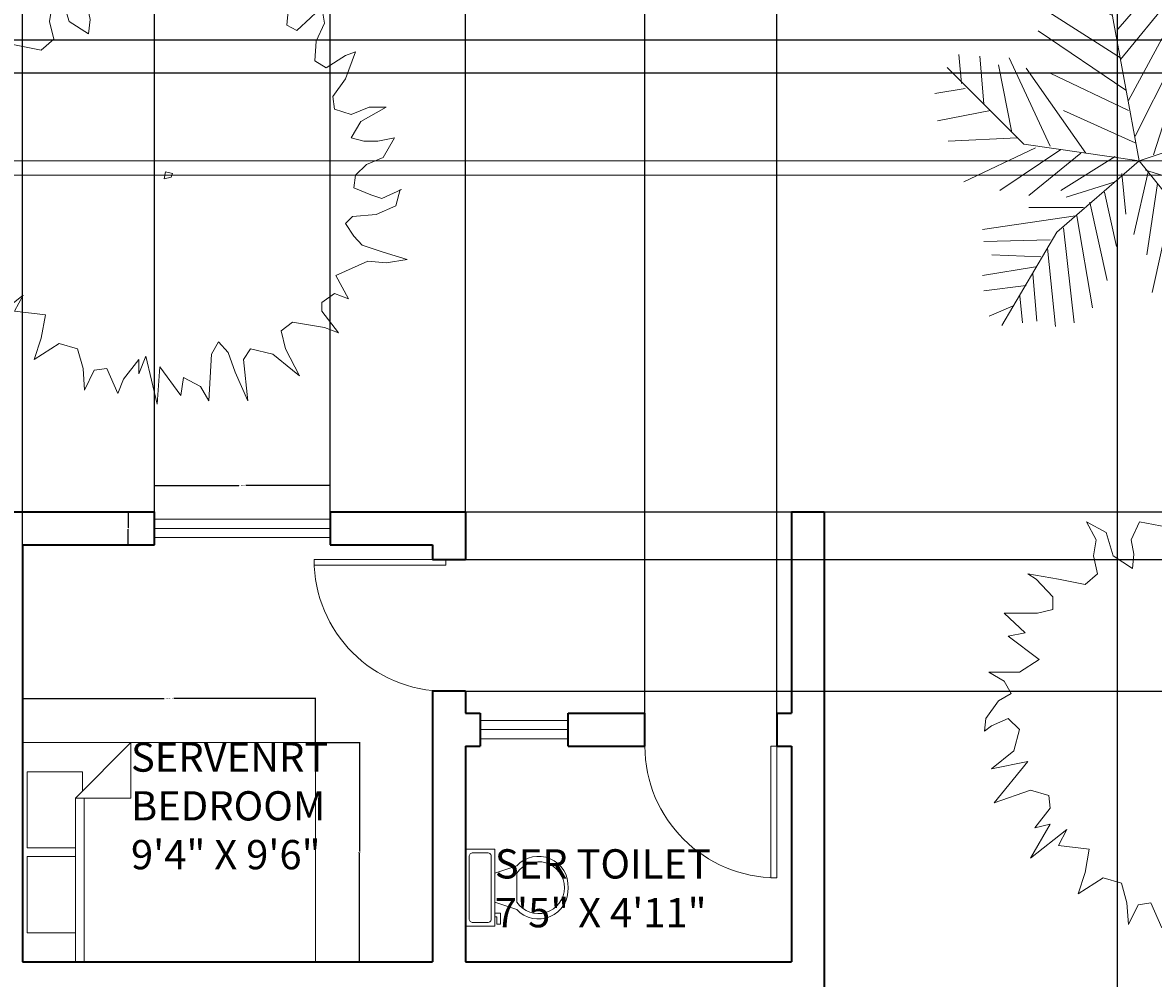
# Model space of a CAD drawing. Units: inches. Extents: x -4843 to -3402, y -164 to 3629.
# Tile 20 of 22: x -4303 to -3994, y 893 to 1154. Entities that reach past the tile are written whole.
import ezdxf

# ---------------------------------------------------------------- set-up
doc = ezdxf.new("R2010")
doc.units = ezdxf.units.IN
for name, color, linetype, lineweight in [('A-ANNO-DIMS', 2, 'Continuous', 18), ('A-AREA-IDEN', 2, 'Continuous', 18), ('C-PROP', 7, 'Continuous', 25), ('doors', 2, 'Continuous', 18), ('furniture', 6, 'Continuous', 18), ('L-PLNT-EDGE', 7, 'Continuous', 18), ('PLANTS', 3, 'Continuous', 13), ('toilets', 5, 'Continuous', 18), ('walls', 7, 'Continuous', 35), ('windows', 1, 'Continuous', 18)]:
    doc.layers.add(name, color=color, linetype=linetype, lineweight=lineweight)
doc.styles.get("Standard").update_dxf_attribs({"font": 'arial.ttf'})
doc.dimstyles.get("Standard").update_dxf_attribs({"dimtxt": 0.18, "dimasz": 0.18, "dimexe": 0.18, "dimexo": 0.0625, "dimgap": 0.09, "dimtad": 0, "dimtih": 1, "dimtoh": 1, "dimdec": 4, "dimzin": 0, "dimdsep": 46, "dimtxsty": 'Standard', "dimcen": 0.09, "dimadec": 0, "dimazin": 0, "dimtfac": 1, "dimtdec": 4, "dimtofl": 0, "dimtmove": 0, "dimatfit": 3, "dimfxl": 1, "dimtolj": 1, "dimtzin": 0, "dimarcsym": 0})

# ---------------------------------------------------------------- blocks, each defined once
blk = doc.blocks.new('window 2')
at = {"layer": 'windows'}
for p, q in [((0, 8.18), (24, 8.18)), ((0, 5.68), (24, 5.68)), ((0, 3.18), (24, 3.18))]:
    blk.add_line(p, q, dxfattribs=at)
for points in [[(0, 10.18), (0, 1.18)], [(24, 1.18), (24, 10.18)]]:
    blk.add_lwpolyline(points, dxfattribs=at)
blk = doc.blocks.new('window 4')
at = {"layer": 'windows'}
for p, q in [((0, 7), (48, 7)), ((0, 4.5), (48, 4.5)), ((0, 2), (48, 2))]:
    blk.add_line(p, q, dxfattribs=at)
for points in [[(0, 0), (0, 9)], [(48, 9), (48, 0)]]:
    blk.add_lwpolyline(points, dxfattribs=at)
blk = doc.blocks.new('*U8')
for p, q in [((0, 0), (0, -6)), ((-40, 0), (-40, -6))]:
    blk.add_line(p, q)
blk.add_lwpolyline([(0, 0), (0, 40), (-1.75, 40), (-1.75, 0)], close=True)
blk.add_arc((0, 0), 40, 90, 180)
blk = doc.blocks.new('*U9')
for p, q in [((-40, 0), (-40, 6)), ((0, 0), (0, 6))]:
    blk.add_line(p, q)
blk.add_lwpolyline([(0, 0), (0, -40), (-1.75, -40), (-1.75, 0)], close=True)
blk.add_arc((0, 0), 40, 180, 270)
blk = doc.blocks.new('Bed - Queen')
for p, q in [((0, -80.00003), (0, 0)), ((0, 0), (59.99999, 0)), ((59.99999, 0), (59.99999, -80.00003)), ((7.99999, -1.2), (28.79998, -1.2)), ((7.99999, -14.4), (7.99999, -1.2)), ((28.79998, -1.2), (28.79998, -14.4)), ((31.19999, -1.2), (51.99999, -1.2)), ((31.19999, -14.4), (31.19999, -1.2)), ((51.99999, -1.2), (51.99999, -16.4)), ((0, -14.4), (44.8, -14.4)), ((59.99999, -29.6), (44.8, -14.4)), ((44.8, -14.4), (44.8, -29.6)), ((44.8, -16.8), (0, -16.8)), ((51.99999, -16.4), (46.79936, -16.4)), ((44.8, -29.6), (59.99999, -29.6)), ((59.99999, -80.00003), (0, -80.00003))]:
    blk.add_line(p, q)
blk = doc.blocks.new('*U31')
for p, q in [((241.3, -152.4), (241.3, -50.8)), ((-254, -215.9), (-203.2, -215.9)), ((-254, -241.3), (-254, -215.9)), ((-203.2, -215.9), (-203.2, -203.2)), ((-177.8, -203.2), (-177.8, -241.3)), ((-101.6, -203.2), (-152.4, -355.6)), ((101.6, -203.2), (152.4, -355.6)), ((-177.8, -241.3), (-254, -241.3)), ((101.6, -355.6), (-101.6, -355.6))]:
    blk.add_line(p, q)
blk.add_lwpolyline([(266.7, -203.2), (266.7, 0), (-266.7, 0), (-266.7, -203.2)], close=True)
for points in [[(-241.3, -50.8), (-241.3, -152.4)], [(215.9, -25.4), (-215.9, -25.4)], [(-215.9, -177.8), (215.9, -177.8)]]:
    blk.add_lwpolyline(points)
for centre, radius, start, end in [((-219.075, -47.625), 22.45064, 81.8699, 188.1301), ((219.075, -47.625), 22.45064, 351.8699, 98.1301), ((-219.075, -155.575), 22.45064, 171.869898, 278.1301), ((219.075, -155.575), 22.45064, 261.8699, 8.1301), ((-12.12088, -505.93752), 205.61935, 133.01722, 273.38), ((0.94996, -504.77674), 181.02486, 124.50543, 269.7), ((-0.94742, -504.77674), 181.02486, 270.3, 55.4946), ((12.12342, -505.93752), 205.61935, 266.62, 46.9828)]:
    blk.add_arc(centre, radius, start, end)
blk = doc.blocks.new('*U33')
for p, q in [((-258.7244, 1362.456), (-332.3336, 1421.4348)), ((0, 0), (-266.7, 1447.8)), ((-231.1146, 1315.2628), (-166.7002, 1421.4348)), ((-221.9198, 1197.3052), (-433.5526, 1338.8594)), ((-194.31, 1102.9442), (-65.4812, 1256.284)), ((-185.1152, 1008.5578), (-553.1612, 1185.4942)), ((-148.3106, 914.1968), (118.5418, 1220.9018)), ((-129.8956, 701.8528), (265.7602, 1185.4942)), ((-129.8956, 713.6638), (-626.7704, 1032.1544)), ((-74.7014, 418.7444), (219.7608, 961.39)), ((-93.091, 489.5342), (-700.3796, 902.3858)), ((685.8, 228.6), (1219.2, 914.4)), ((689.0258, 230.0224), (790.2448, 914.1968)), ((983.4626, 867.0036), (1066.2666, 725.4494)), ((1121.4862, 925.9824), (1149.0706, 831.6214)), ((412.9786, 147.447), (587.8068, 796.2392)), ((560.197, 182.8292), (698.2206, 819.8358)), ((891.4384, 831.6214), (946.658, 572.1096)), ((-1234.059, 536.7274), (-1252.4486, 737.2604)), ((-1105.2302, 725.4494), (-1077.6458, 395.1732)), ((-902.8176, 713.6638), (-617.5756, 100.2538)), ((808.6344, 784.4282), (827.0494, 418.7444)), ((1112.2914, 760.8316), (1296.3144, 784.4282)), ((-800.1, 114.3), (-1333.5, 647.7)), ((-976.4268, 666.4706), (-884.4026, 194.6402)), ((-369.1382, 53.086), (-783.1836, 642.874)), ((-28.6766, 171.0436), (228.9556, 678.2816)), ((256.5654, 88.4682), (449.7832, 666.4706)), ((1029.462, 654.685), (1241.0948, 631.0884)), ((-617.5756, 607.4918), (-74.7014, 347.98)), ((100.1268, 41.275), (284.1498, 619.2774)), ((-1206.4492, 501.3198), (-1418.082, 465.9376)), ((919.0482, 501.3198), (1222.6798, 454.152)), ((845.439, 418.7444), (1241.0948, 277.1902)), ((-1031.621, 347.98), (-1399.667, 277.1902)), ((-525.5514, 347.98), (-28.6766, 123.8504)), ((753.4148, 312.5978), (1222.6798, 159.2326)), ((-847.598, 159.2326), (-1326.0578, 135.636)), ((0, 0), (685.8, 228.6)), ((615.4166, 194.6402), (1185.8752, 41.275)), ((-718.7946, 88.4682), (-1215.644, -147.447)), ((0, 0), (-800.1, 114.3)), ((284.1498, 88.4682), (781.0246, -147.447)), ((458.978, 147.447), (891.4384, -88.4682)), ((-543.9664, 76.6572), (-967.2066, -206.4512)), ((-405.9428, 53.086), (-764.794, -241.8334)), ((0, 0), (-571.5, -495.3)), ((-166.7002, 29.4894), (-543.9664, -206.4512)), ((0, 0), (457.2, -571.5)), ((164.5412, 41.275), (661.416, -218.2368)), ((63.3222, -76.6826), (-37.8714, -513.1308)), ((44.9326, -64.897), (615.4166, -241.8334)), ((-166.7002, -147.447), (-507.1618, -253.619)), ((-120.7008, -88.4682), (-93.091, -371.5766)), ((-240.3094, -218.2368), (-157.5054, -595.7062)), ((127.7366, -159.258), (54.1274, -654.685)), ((192.151, -230.0224), (817.8292, -371.5766)), ((-341.5284, -289.0012), (-221.9198, -831.6214)), ((228.9556, -289.0012), (90.932, -914.1968)), ((-442.7474, -383.3876), (-1086.8406, -477.7486)), ((-387.5278, -324.4088), (-764.794, -324.4088)), ((-433.5526, -383.3876), (-323.1134, -1020.3688)), ((311.7596, -383.3876), (937.4378, -477.7486)), ((-525.5514, -465.963), (-451.9422, -1126.5408)), ((357.759, -430.5554), (164.5412, -1020.3688)), ((-617.5756, -548.5384), (-1077.6458, -560.324)), ((-571.5, -495.3), (-952.5, -1143)), ((412.9786, -501.3452), (919.0482, -583.9206)), ((-635.9652, -607.5172), (-580.771, -1150.1374)), ((458.978, -572.1096), (210.5406, -1161.923)), ((457.2, -571.5), (685.8, -1333.5)), ((468.1982, -572.1096), (1029.462, -737.2604)), ((-681.9646, -666.496), (-1022.4262, -654.685)), ((486.5878, -642.8994), (983.4626, -843.4324)), ((-718.7946, -737.2604), (-1086.8406, -796.2392)), ((-737.1842, -784.4536), (-709.5744, -1114.7298)), ((514.1976, -772.6426), (403.7838, -1138.3264)), ((541.8074, -831.6214), (992.6574, -1032.1544)), ((-783.1836, -867.029), (-1077.6458, -902.4112)), ((-829.2084, -937.7934), (-810.7934, -1126.5408)), ((-875.2078, -1008.5832), (-1040.8412, -1079.3476)), ((578.612, -961.39), (495.7826, -1232.7128)), ((578.612, -973.1756), (873.0488, -1138.3264)), ((624.6114, -1161.923), (587.8068, -1291.6916)), ((624.6114, -1102.9442), (781.0246, -1209.1162)), ((679.8056, -1268.095), (716.6102, -1291.6916))]:
    blk.add_line(p, q)
blk = doc.blocks.new('*U34')
for points in [[(0, 1540.256), (-77.4954, 1428.4452), (-106.5784, 1341.501), (-135.636, 1217.295), (-155.0162, 1167.6126), (-280.9748, 1291.8186), (-474.7514, 1329.0804), (-532.892, 1204.8744), (-513.5118, 1105.5096), (-523.1892, 1006.1194), (-658.8506, 1093.089), (-707.2884, 1254.5568), (-842.9244, 1329.0804), (-775.1064, 1204.8744), (-794.4866, 1093.089), (-765.429, 968.8576), (-852.6272, 894.334), (-1036.701, 931.5958), (-1249.8832, 968.8576), (-1191.7426, 931.5958), (-1075.4614, 807.3898), (-1075.4614, 720.4456), (-1182.0398, 695.6044), (-1414.5768, 695.6044), (-1269.238, 558.9524), (-1385.5192, 534.1112), (-1172.3624, 372.6434), (-1307.9984, 285.6992), (-1521.1552, 285.6992), (-1414.5768, 223.5962), (-1366.139, 136.652), (-1453.3372, 86.9442), (-1540.5354, -37.2618), (-1550.2382, -124.206), (-1501.775, -86.9442), (-1385.5192, -37.2618), (-1307.9984, -111.7854), (-1346.7588, -260.8326), (-1501.775, -385.064), (-1249.8832, -335.3816), (-1482.3948, -621.0554), (-1230.503, -534.1112), (-1104.5444, -571.373), (-1094.8416, -658.3172), (-1201.42, -794.9692), (-1094.8416, -770.128), (-1230.503, -1006.1194), (-978.5858, -807.3898), (-1036.701, -919.1752), (-823.5442, -944.0164), (-852.6272, -1105.4842), (-901.065, -1254.5568), (-726.6686, -1142.746), (-600.71, -1180.0078), (-561.9496, -1316.6598), (-552.2722, -1465.707), (-484.4542, -1329.0804), (-397.2306, -1316.6598), (-319.7352, -1490.5482), (-280.9748, -1391.1834), (-174.3964, -1254.5568), (-174.3964, -1353.9216), (-125.9586, -1229.7156), (-48.4378, -1565.0718), (-29.0576, -1304.2392), (116.2812, -1502.9688), (135.6614, -1378.7628), (251.9172, -1440.8658), (310.0578, -1540.2306), (329.438, -1217.295), (377.8758, -1130.3254), (445.6938, -1204.8744), (494.157, -1341.501), (581.3552, -1540.2306), (552.2722, -1254.5568), (600.71, -1180.0078), (755.7516, -1217.295), (891.3876, -1329.0804), (939.8254, -1366.3422), (842.9498, -1180.0078), (813.8668, -1055.8018), (891.3876, -993.6988), (1114.2472, -1030.9606), (1211.1228, -1068.2224), (1094.867, -919.1752), (1094.867, -857.0722), (1182.0652, -794.9692), (1278.9408, -832.231), (1191.7426, -670.7378), (1414.6022, -571.373), (1540.5608, -583.7936), (1685.8996, -558.9524), (1521.1806, -509.27), (1375.8418, -459.5876), (1317.7012, -397.4846), (1259.5606, -310.515), (1308.0238, -260.8326), (1472.7174, -248.412), (1608.3788, -186.309), (1637.4364, -74.5236)], [(1647.1392, -74.5236), (1511.4778, -136.6266), (1433.9824, -111.7854), (1317.7012, -62.103), (1327.404, 24.8412), (1404.8994, 99.3648), (1521.1806, 149.0726), (1598.676, 285.6992), (1482.4202, 260.858), (1385.5192, 260.858), (1298.321, 285.6992), (1366.139, 397.4846), (1472.7174, 459.5876), (1540.5608, 496.8494), (1424.2796, 496.8494), (1298.321, 447.167), (1182.0652, 484.4288), (1172.3624, 571.3984), (1259.5606, 695.6044), (1327.404, 881.9134), (1259.5606, 857.0722), (1123.9246, 770.128), (1046.4038, 819.8104), (1056.1066, 956.437), (1114.2472, 1080.6684), (1094.867, 1192.4538), (1017.3462, 1117.9302), (920.4452, 1030.9606), (852.6272, 1068.2478), (862.33, 1167.6126), (901.0904, 1341.501), (794.512, 1254.5568), (678.2308, 1192.4538), (716.9912, 1291.8186), (726.6686, 1552.6766), (629.793, 1378.7628), (474.7768, 1291.8186), (455.3966, 1465.7324), (329.438, 1291.8186), (184.0992, 1465.7324), (135.6614, 1353.9216), (0, 1540.256)]]:
    blk.add_lwpolyline(points)
blk.add_lwpolyline([(9.7028, 49.6824), (0, 0), (48.4378, 12.4206), (58.1406, 37.2618)], close=True)
blk = doc.blocks.new('*D42')
at = {"layer": 'A-ANNO-DIMS', "color": 0, "lineweight": -2, "transparency": 16777216}
for p, q in [((-4266.78, 1020.42), (-4266.78, 1027.73)), ((-4266.6, 1027.55), (-4243.72, 1027.55)), ((-4218.96, 1027.55), (-4241.85, 1027.55)), ((-4218.78, 1020.42), (-4218.78, 1027.73))]:
    blk.add_line(p, q, dxfattribs=at)
at = {"layer": 'A-ANNO-DIMS', "color": 0, "transparency": 16777216}
for points in [[(-4266.6, 1027.58), (-4266.6, 1027.52), (-4266.78, 1027.55)], [(-4218.96, 1027.58), (-4218.96, 1027.52), (-4218.78, 1027.55)]]:
    blk.add_solid(points, dxfattribs=at)
at = {"layer": 'Defpoints', "color": 0, "transparency": 16777216}
for p in [(-4266.78, 1027.55), (-4266.78, 1020.35), (-4218.78, 1020.35)]:
    blk.add_point(p, dxfattribs=at)
at = {"layer": 'A-ANNO-DIMS', "color": 0, "transparency": 16777216, "insert": (-4242.78, 1027.55), "char_height": 0.18, "attachment_point": 5}
blk.add_mtext('\\A1;WINDOW D 48', dxfattribs=at)
blk = doc.blocks.new('*D43')
at = {"layer": 'A-ANNO-DIMS', "color": 0, "lineweight": -2, "transparency": 16777216}
for p, q in [((-4266.85, 1020.35), (-4274.16, 1020.35)), ((-4273.98, 1020.17), (-4273.98, 1016.04)), ((-4273.98, 1011.53), (-4273.98, 1015.67)), ((-4266.85, 1011.35), (-4274.16, 1011.35))]:
    blk.add_line(p, q, dxfattribs=at)
at = {"layer": 'A-ANNO-DIMS', "color": 0, "transparency": 16777216}
for points in [[(-4274.01, 1020.17), (-4273.95, 1020.17), (-4273.98, 1020.35)], [(-4274.01, 1011.53), (-4273.95, 1011.53), (-4273.98, 1011.35)]]:
    blk.add_solid(points, dxfattribs=at)
at = {"layer": 'Defpoints', "color": 0, "transparency": 16777216}
for p in [(-4266.78, 1020.35), (-4273.98, 1011.35), (-4266.78, 1011.35)]:
    blk.add_point(p, dxfattribs=at)
at = {"layer": 'A-ANNO-DIMS', "color": 0, "transparency": 16777216, "insert": (-4273.98, 1015.85), "char_height": 0.18, "attachment_point": 5}
blk.add_mtext('\\A1;9', dxfattribs=at)
blk = doc.blocks.new('*D44')
at = {"layer": 'A-ANNO-DIMS', "color": 0, "lineweight": -2, "transparency": 16777216}
for p, q in [((-4302.78, 957.42), (-4302.78, 969.53)), ((-4302.6, 969.35), (-4264.09, 969.35)), ((-4222.96, 969.35), (-4261.48, 969.35)), ((-4222.78, 957.42), (-4222.78, 969.53))]:
    blk.add_line(p, q, dxfattribs=at)
at = {"layer": 'A-ANNO-DIMS', "color": 0, "transparency": 16777216}
for points in [[(-4302.6, 969.38), (-4302.6, 969.32), (-4302.78, 969.35)], [(-4222.96, 969.38), (-4222.96, 969.32), (-4222.78, 969.35)]]:
    blk.add_solid(points, dxfattribs=at)
at = {"layer": 'Defpoints', "color": 0, "transparency": 16777216}
for p in [(-4302.78, 969.35), (-4302.78, 957.35), (-4222.78, 957.35)]:
    blk.add_point(p, dxfattribs=at)
at = {"layer": 'A-ANNO-DIMS', "color": 0, "transparency": 16777216, "insert": (-4262.78, 969.35), "char_height": 0.18, "attachment_point": 5}
blk.add_mtext('\\A1;QUEEN BED 80 TYP.', dxfattribs=at)
blk = doc.blocks.new('*D45')
at = {"layer": 'A-ANNO-DIMS', "color": 0, "lineweight": -2, "transparency": 16777216}
for p, q in [((-4222.72, 957.35), (-4210.6, 957.35)), ((-4210.78, 957.17), (-4210.78, 927.54)), ((-4210.78, 897.53), (-4210.78, 927.17)), ((-4222.72, 897.35), (-4210.6, 897.35))]:
    blk.add_line(p, q, dxfattribs=at)
at = {"layer": 'A-ANNO-DIMS', "color": 0, "transparency": 16777216}
for points in [[(-4210.81, 957.17), (-4210.75, 957.17), (-4210.78, 957.35)], [(-4210.81, 897.53), (-4210.75, 897.53), (-4210.78, 897.35)]]:
    blk.add_solid(points, dxfattribs=at)
at = {"layer": 'Defpoints', "color": 0, "transparency": 16777216}
for p in [(-4222.78, 957.35), (-4210.78, 957.35), (-4222.78, 897.35)]:
    blk.add_point(p, dxfattribs=at)
at = {"layer": 'A-ANNO-DIMS', "color": 0, "transparency": 16777216, "insert": (-4210.78, 927.35), "char_height": 0.18, "attachment_point": 5}
blk.add_mtext('\\A1;60 TYP.', dxfattribs=at)
blk = doc.blocks.new('*D60')
at = {"layer": 'A-ANNO-DIMS', "color": 0, "lineweight": -2, "transparency": 16777216}
for p, q in [((-4723.78, 1149.42), (-4723.78, 1392.95)), ((-4723.6, 1392.77), (-4333.07, 1392.77)), ((-3941.96, 1392.77), (-4332.5, 1392.77)), ((-3941.78, 1149.42), (-3941.78, 1392.95))]:
    blk.add_line(p, q, dxfattribs=at)
at = {"layer": 'A-ANNO-DIMS', "color": 0, "transparency": 16777216}
for points in [[(-4723.6, 1392.8), (-4723.6, 1392.74), (-4723.78, 1392.77)], [(-3941.96, 1392.8), (-3941.96, 1392.74), (-3941.78, 1392.77)]]:
    blk.add_solid(points, dxfattribs=at)
at = {"layer": 'Defpoints', "color": 0, "transparency": 16777216}
for p in [(-3941.78, 1392.77), (-4723.78, 1149.35), (-3941.78, 1149.35)]:
    blk.add_point(p, dxfattribs=at)
at = {"layer": 'A-ANNO-DIMS', "color": 0, "transparency": 16777216, "insert": (-4332.78, 1392.77), "char_height": 0.18, "attachment_point": 5}
blk.add_mtext('\\A1;782', dxfattribs=at)
blk = doc.blocks.new('*D72')
at = {"layer": 'A-ANNO-DIMS', "color": 0, "lineweight": -2, "transparency": 16777216}
for p, q in [((-4302.78, 1011.42), (-4302.78, 1392.95)), ((-4302.6, 1392.77), (-4285, 1392.77)), ((-4266.96, 1392.77), (-4284.56, 1392.77)), ((-4266.78, 1020.42), (-4266.78, 1392.95))]:
    blk.add_line(p, q, dxfattribs=at)
at = {"layer": 'A-ANNO-DIMS', "color": 0, "transparency": 16777216}
for points in [[(-4302.6, 1392.8), (-4302.6, 1392.74), (-4302.78, 1392.77)], [(-4266.96, 1392.8), (-4266.96, 1392.74), (-4266.78, 1392.77)]]:
    blk.add_solid(points, dxfattribs=at)
at = {"layer": 'Defpoints', "color": 0, "transparency": 16777216}
for p in [(-4266.78, 1392.77), (-4266.78, 1020.35), (-4302.78, 1011.35)]:
    blk.add_point(p, dxfattribs=at)
at = {"layer": 'A-ANNO-DIMS', "color": 0, "transparency": 16777216, "insert": (-4284.78, 1392.77), "char_height": 0.18, "attachment_point": 5}
blk.add_mtext('\\A1;36', dxfattribs=at)
blk = doc.blocks.new('*D77')
at = {"layer": 'A-ANNO-DIMS', "color": 0, "lineweight": -2, "transparency": 16777216}
for p, q in [((-4181.72, 1020.35), (-3828.78, 1020.35)), ((-3828.96, 1020.17), (-3828.96, 1014.04)), ((-3828.96, 1007.53), (-3828.96, 1013.67)), ((-4181.72, 1007.35), (-3828.78, 1007.35))]:
    blk.add_line(p, q, dxfattribs=at)
at = {"layer": 'A-ANNO-DIMS', "color": 0, "transparency": 16777216}
for points in [[(-3828.99, 1020.17), (-3828.93, 1020.17), (-3828.96, 1020.35)], [(-3828.99, 1007.53), (-3828.93, 1007.53), (-3828.96, 1007.35)]]:
    blk.add_solid(points, dxfattribs=at)
at = {"layer": 'Defpoints', "color": 0, "transparency": 16777216}
for p in [(-4181.78, 1020.35), (-4181.78, 1007.35), (-3828.96, 1007.35)]:
    blk.add_point(p, dxfattribs=at)
at = {"layer": 'A-ANNO-DIMS', "color": 0, "transparency": 16777216, "insert": (-3828.96, 1013.85), "char_height": 0.18, "attachment_point": 5}
blk.add_mtext('\\A1;13', dxfattribs=at)
blk = doc.blocks.new('*D78')
at = {"layer": 'A-ANNO-DIMS', "color": 0, "lineweight": -2, "transparency": 16777216}
for p, q in [((-4181.72, 1007.35), (-3828.78, 1007.35)), ((-3828.96, 1007.17), (-3828.96, 989.54)), ((-3828.96, 971.53), (-3828.96, 989.17)), ((-4181.72, 971.35), (-3828.78, 971.35))]:
    blk.add_line(p, q, dxfattribs=at)
at = {"layer": 'A-ANNO-DIMS', "color": 0, "transparency": 16777216}
for points in [[(-3828.99, 1007.17), (-3828.93, 1007.17), (-3828.96, 1007.35)], [(-3828.99, 971.53), (-3828.93, 971.53), (-3828.96, 971.35)]]:
    blk.add_solid(points, dxfattribs=at)
at = {"layer": 'Defpoints', "color": 0, "transparency": 16777216}
for p in [(-4181.78, 1007.35), (-4181.78, 971.35), (-3828.96, 971.35)]:
    blk.add_point(p, dxfattribs=at)
at = {"layer": 'A-ANNO-DIMS', "color": 0, "transparency": 16777216, "insert": (-3828.96, 989.35), "char_height": 0.18, "attachment_point": 5}
blk.add_mtext('\\A1;36', dxfattribs=at)
blk = doc.blocks.new('*D79')
at = {"layer": 'A-ANNO-DIMS', "color": 0, "lineweight": -2, "transparency": 16777216}
for p, q in [((-4132.78, 965.42), (-4132.78, 1392.95)), ((-4132.6, 1392.77), (-4115, 1392.77)), ((-4096.96, 1392.77), (-4114.56, 1392.77)), ((-4096.78, 965.42), (-4096.78, 1392.95))]:
    blk.add_line(p, q, dxfattribs=at)
at = {"layer": 'A-ANNO-DIMS', "color": 0, "transparency": 16777216}
for points in [[(-4132.6, 1392.8), (-4132.6, 1392.74), (-4132.78, 1392.77)], [(-4096.96, 1392.8), (-4096.96, 1392.74), (-4096.78, 1392.77)]]:
    blk.add_solid(points, dxfattribs=at)
at = {"layer": 'Defpoints', "color": 0, "transparency": 16777216}
for p in [(-4096.78, 1392.77), (-4132.78, 965.35), (-4096.78, 965.35)]:
    blk.add_point(p, dxfattribs=at)
at = {"layer": 'A-ANNO-DIMS', "color": 0, "transparency": 16777216, "insert": (-4114.78, 1392.77), "char_height": 0.18, "attachment_point": 5}
blk.add_mtext('\\A1;36', dxfattribs=at)
blk = doc.blocks.new('*D80')
at = {"layer": 'A-ANNO-DIMS', "color": 0, "lineweight": -2, "transparency": 16777216}
for p, q in [((-4218.78, 1020.42), (-4218.78, 1392.95)), ((-4218.6, 1392.77), (-4200.5, 1392.77)), ((-4181.96, 1392.77), (-4200.06, 1392.77)), ((-4181.78, 1020.42), (-4181.78, 1392.95))]:
    blk.add_line(p, q, dxfattribs=at)
at = {"layer": 'A-ANNO-DIMS', "color": 0, "transparency": 16777216}
for points in [[(-4218.6, 1392.8), (-4218.6, 1392.74), (-4218.78, 1392.77)], [(-4181.96, 1392.8), (-4181.96, 1392.74), (-4181.78, 1392.77)]]:
    blk.add_solid(points, dxfattribs=at)
at = {"layer": 'Defpoints', "color": 0, "transparency": 16777216}
for p in [(-4181.78, 1392.77), (-4218.78, 1020.35), (-4181.78, 1020.35)]:
    blk.add_point(p, dxfattribs=at)
at = {"layer": 'A-ANNO-DIMS', "color": 0, "transparency": 16777216, "insert": (-4200.28, 1392.77), "char_height": 0.18, "attachment_point": 5}
blk.add_mtext('\\A1;37', dxfattribs=at)
blk = doc.blocks.new('*D81')
at = {"layer": 'A-ANNO-DIMS', "color": 0, "lineweight": -2, "transparency": 16777216}
for p, q in [((-4332.78, 86.42), (-4332.78, 1392.95)), ((-4332.6, 1392.77), (-4168.61, 1392.77)), ((-4003.86, 1392.77), (-4167.86, 1392.77)), ((-4003.68, 86.42), (-4003.68, 1392.95))]:
    blk.add_line(p, q, dxfattribs=at)
at = {"layer": 'A-ANNO-DIMS', "color": 0, "transparency": 16777216}
for points in [[(-4332.6, 1392.8), (-4332.6, 1392.74), (-4332.78, 1392.77)], [(-4003.86, 1392.8), (-4003.86, 1392.74), (-4003.68, 1392.77)]]:
    blk.add_solid(points, dxfattribs=at)
at = {"layer": 'Defpoints', "color": 0, "transparency": 16777216}
for p in [(-4003.68, 1392.77), (-4332.78, 86.35), (-4003.68, 86.35)]:
    blk.add_point(p, dxfattribs=at)
at = {"layer": 'A-ANNO-DIMS', "color": 0, "transparency": 16777216, "insert": (-4168.23, 1392.77), "char_height": 0.18, "attachment_point": 5}
blk.add_mtext('\\A1;329.1', dxfattribs=at)

msp = doc.modelspace()

# ---------------------------------------------------------------- linework, layer by layer
at = {"layer": 'C-PROP'}
for p, q in [((-4723.78, 1149.35), (-3941.78, 1149.35)), ((-4714.78, 1140.35), (-3950.78, 1140.35))]:
    msp.add_line(p, q, dxfattribs=at)
at = {"layer": 'L-PLNT-EDGE'}
for p, q in [((-4696.78, 1116.35), (-3974.78, 1116.35)), ((-4696.78, 1112.35), (-3978.78, 1112.35))]:
    msp.add_line(p, q, dxfattribs=at)
at = {"layer": 'walls'}
for p, q in [((-4342.78, 1020.35), (-4266.78, 1020.35)), ((-4218.78, 1020.35), (-4181.78, 1020.35)), ((-4181.78, 1020.35), (-4181.78, 1007.35)), ((-4092.78, 1020.35), (-4092.78, 965.35)), ((-4092.78, 1020.35), (-4083.78, 1020.35)), ((-4083.78, 1020.35), (-4083.78, 888.35)), ((-4302.78, 1011.35), (-4302.78, 897.35)), ((-4302.78, 1011.35), (-4266.78, 1011.35)), ((-4218.78, 1011.35), (-4190.78, 1011.35)), ((-4190.78, 1011.35), (-4190.78, 1007.35)), ((-4190.78, 971.35), (-4190.78, 897.35)), ((-4181.78, 971.35), (-4181.78, 965.35)), ((-4181.78, 965.35), (-4177.78, 965.35)), ((-4153.78, 965.35), (-4132.78, 965.35)), ((-4096.78, 965.35), (-4092.78, 965.35)), ((-4181.78, 956.35), (-4177.78, 956.35)), ((-4181.78, 956.35), (-4181.78, 897.35)), ((-4153.78, 956.35), (-4132.78, 956.35)), ((-4096.78, 956.35), (-4092.78, 956.35)), ((-4092.78, 956.35), (-4092.78, 897.35)), ((-4302.78, 897.35), (-4190.78, 897.35)), ((-4181.78, 897.35), (-4092.78, 897.35))]:
    msp.add_line(p, q, dxfattribs=at)
for points in [[(-4266.78, 1011.35), (-4266.78, 1020.35)], [(-4218.78, 1020.35), (-4218.78, 1011.35)], [(-4190.78, 1007.35), (-4181.78, 1007.35)], [(-4181.78, 971.35), (-4190.78, 971.35)], [(-4177.78, 965.35), (-4177.78, 956.35)], [(-4153.78, 956.35), (-4153.78, 965.35)], [(-4132.78, 956.35), (-4132.78, 965.35)], [(-4096.78, 965.35), (-4096.78, 956.35)]]:
    msp.add_lwpolyline(points, dxfattribs=at)

# ---------------------------------------------------------------- block references
at = {"layer": 'doors', "xscale": 0.9, "yscale": 0.9, "zscale": 0.9, "rotation": 90}
msp.add_blockref('*U8', (-4187.18, 1007.35), dxfattribs=at)
at = {"layer": 'doors', "xscale": 0.9, "yscale": 0.9, "zscale": 0.9}
msp.add_blockref('*U9', (-4096.78, 956.35), dxfattribs=at)
at = {"layer": 'furniture', "rotation": 90}
msp.add_blockref('Bed - Queen', (-4302.78, 897.35), dxfattribs=at)
at = {"layer": 'PLANTS', "xscale": 0.0393700787401575, "yscale": 0.0393700787401575, "zscale": 0.0393700787401575}
for name, p in [('*U34', (-4264.15, 1111.38)), ('*U33', (-3997.76, 1116.35)), ('*U34', (-3978.97, 965.32))]:
    msp.add_blockref(name, p, dxfattribs=at)
at = {"layer": 'toilets', "xscale": 0.0393700787401575, "yscale": 0.0393700787401575, "zscale": 0.0393700787401575, "rotation": 90}
msp.add_blockref('*U31', (-4181.78, 917.65), dxfattribs=at)
at = {"layer": 'windows', "rotation": 180}
msp.add_blockref('window 4', (-4218.78, 1020.35), dxfattribs=at)
at = {"layer": 'windows'}
msp.add_blockref('window 2', (-4177.78, 955.17), dxfattribs=at)

# ---------------------------------------------------------------- texts
at = {"layer": 'A-AREA-IDEN', "char_height": 8, "attachment_point": 1}
for s, insert in [('SERVENRT BEDROOM \\P9\'4" X 9\'6"', (-4273.18, 957.35)), ('SER TOILET \\P7\'5" X 4\'11"', (-4173.78, 928.15))]:
    msp.add_mtext_dynamic_manual_height_columns(s, width=66.873, gutter_width=60, heights=[0], dxfattribs=dict(at, insert=insert))

# ---------------------------------------------------------------- dimensions: what is measured, and where the dimension line sits
at = {"layer": 'A-ANNO-DIMS'}
for base, p1, p2, override, picture, middle in [((-3941.78, 1392.77), (-4723.78, 1149.35), (-3941.78, 1149.35), {"dimdec": 0, "dimlfac": 1, "dimrnd": 0, "dimzin": 0, "dimdsep": 46, "dimlunit": 2}, '*D60', (-4332.78, 1392.77)), ((-4003.68, 1392.77), (-4332.78, 86.35), (-4003.68, 86.35), {"dimdec": 1, "dimlfac": 1, "dimrnd": 0, "dimzin": 0, "dimdsep": 46, "dimlunit": 2}, '*D81', (-4168.23, 1392.77)), ((-4266.78, 1392.77), (-4302.78, 1011.35), (-4266.78, 1020.35), {"dimdec": 0, "dimlfac": 1, "dimrnd": 0, "dimzin": 0, "dimdsep": 46, "dimlunit": 2}, '*D72', (-4284.78, 1392.77)), ((-4181.78, 1392.77), (-4218.78, 1020.35), (-4181.78, 1020.35), {"dimdec": 0, "dimlfac": 1, "dimrnd": 0, "dimzin": 0, "dimdsep": 46, "dimlunit": 2}, '*D80', (-4200.28, 1392.77)), ((-4096.78, 1392.77), (-4132.78, 965.35), (-4096.78, 965.35), {"dimdec": 0, "dimlfac": 1, "dimrnd": 0, "dimzin": 0, "dimdsep": 46, "dimlunit": 2}, '*D79', (-4114.78, 1392.77))]:
    dim = msp.add_linear_dim(base=base, p1=p1, p2=p2, dimstyle='Standard', override=override, dxfattribs=at)
    dim.commit()
    dim.dimension.update_dxf_attribs({"geometry": picture, "text_midpoint": middle})
for base, p1, p2, angle, text, picture, middle in [((-4266.78, 1027.55), (-4218.78, 1020.35), (-4266.78, 1020.35), 180, 'WINDOW D <>', '*D42', (-4242.78, 1027.55)), ((-4302.78, 969.35), (-4222.78, 957.35), (-4302.78, 957.35), 180, 'QUEEN BED <> TYP.', '*D44', (-4262.78, 969.35)), ((-4210.78, 957.35), (-4222.78, 897.35), (-4222.78, 957.35), 90, '<> TYP.', '*D45', (-4210.78, 927.35))]:
    dim = msp.add_linear_dim(base=base, p1=p1, p2=p2, angle=angle, text=text, dimstyle='Standard', override={"dimdec": 0, "dimlfac": 1, "dimrnd": 0, "dimzin": 0, "dimdsep": 46, "dimlunit": 2}, dxfattribs=at)
    dim.commit()
    dim.dimension.update_dxf_attribs({"geometry": picture, "text_midpoint": middle})
for base, p1, p2, angle, picture, middle in [((-4273.98, 1011.35), (-4266.78, 1020.35), (-4266.78, 1011.35), 270, '*D43', (-4273.98, 1015.85)), ((-3828.96, 1007.35), (-4181.78, 1020.35), (-4181.78, 1007.35), 90, '*D77', (-3828.96, 1013.85)), ((-3828.96, 971.35), (-4181.78, 1007.35), (-4181.78, 971.35), 90, '*D78', (-3828.96, 989.35))]:
    dim = msp.add_linear_dim(base=base, p1=p1, p2=p2, angle=angle, dimstyle='Standard', override={"dimdec": 0, "dimlfac": 1, "dimrnd": 0, "dimzin": 0, "dimdsep": 46, "dimlunit": 2}, dxfattribs=at)
    dim.commit()
    dim.dimension.update_dxf_attribs({"geometry": picture, "text_midpoint": middle})

doc.saveas('drawing.dxf')
